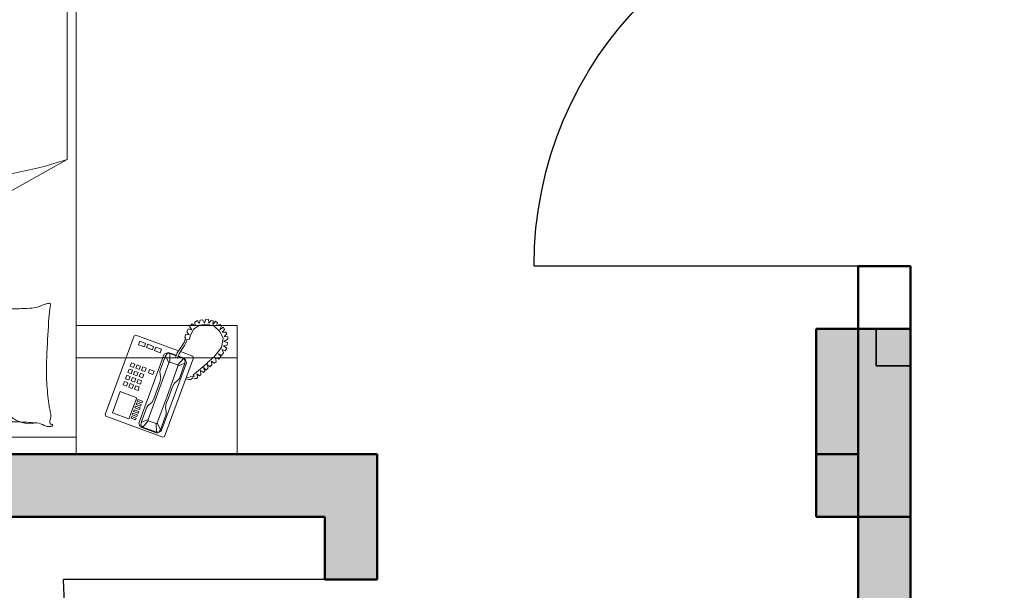
# Model space of a CAD drawing. Units: inches. Extents: x -7 to 1228, y -146 to 1091.
# Tile 75 of 88: x 722 to 816, y 835 to 890. Entities that reach past the tile are written whole.
import ezdxf

# ---------------------------------------------------------------- set-up
doc = ezdxf.new("R2010")
doc.units = ezdxf.units.IN
for name, color, linetype, lineweight in [('A-COLS', 6, 'Continuous', 35), ('A-DOOR', 4, 'Continuous', 25), ('A-FURN', 8, 'Continuous', 18), ('A-WALL', 7, 'Continuous', 50), ('A-WALL-PATT', 251, 'Continuous', 13)]:
    doc.layers.add(name, color=color, linetype=linetype, lineweight=lineweight)
doc.styles.add('DIM_FONT', font='SIMPLEX.shx', dxfattribs={"width": 0.8})

# ---------------------------------------------------------------- blocks, each defined once
blk = doc.blocks.new('A$C4F634EDD')
for p, q in [((0.5, 2.6295), (2.3, 2.6295)), ((2.3, 2.6295), (2.3, 0.5295)), ((2.3, 2.6295), (2.8, 2.6295)), ((2.3, 2.2295), (2.3, 2.6295)), ((2.8, 2.6295), (2.8, 2.2295)), ((0.5, 2.5771), (2.3, 2.5771)), ((2.392, 2.5115), (2.5692, 2.5765)), ((2.5692, 2.5765), (2.574, 2.5743)), ((2.574, 2.5743), (2.6638, 2.3298)), ((2.4946, 2.5331), (2.4985, 2.5445)), ((2.4985, 2.5445), (2.5516, 2.564)), ((2.5062, 2.5454), (2.5004, 2.5392)), ((2.5004, 2.5392), (2.5013, 2.5315)), ((2.5062, 2.5454), (2.5487, 2.561)), ((2.5235, 2.5256), (2.5062, 2.5454)), ((2.5483, 2.5347), (2.5487, 2.561)), ((2.5487, 2.561), (2.5571, 2.56)), ((2.5615, 2.5536), (2.5514, 2.5318)), ((2.5516, 2.564), (2.5637, 2.5584)), ((2.5571, 2.56), (2.5615, 2.5536)), ((2.5615, 2.5536), (2.5791, 2.5058)), ((2.5637, 2.5584), (2.6418, 2.3458)), ((2.3898, 2.5066), (2.392, 2.5115)), ((2.412, 2.5007), (2.4634, 2.5196)), ((2.4634, 2.5196), (2.4875, 2.454)), ((2.4842, 2.5232), (2.47, 2.518)), ((2.47, 2.518), (2.472, 2.5127)), ((2.472, 2.5127), (2.4862, 2.5179)), ((2.4881, 2.5126), (2.4739, 2.5074)), ((2.4862, 2.5179), (2.4842, 2.5232)), ((2.4901, 2.5073), (2.4881, 2.5126)), ((2.5734, 2.3187), (2.4946, 2.5331)), ((2.5013, 2.5315), (2.5188, 2.4836)), ((2.5013, 2.5315), (2.5231, 2.5214)), ((2.5231, 2.5214), (2.5235, 2.5256)), ((2.5523, 2.4417), (2.5231, 2.5214)), ((2.5483, 2.5347), (2.5235, 2.5256)), ((2.5514, 2.5318), (2.5483, 2.5347)), ((2.5807, 2.4521), (2.5514, 2.5318)), ((2.4795, 2.2621), (2.3898, 2.5066)), ((2.4361, 2.4352), (2.412, 2.5007)), ((2.4739, 2.5074), (2.4759, 2.502)), ((2.4759, 2.502), (2.4901, 2.5073)), ((2.492, 2.5019), (2.4778, 2.4967)), ((2.4778, 2.4967), (2.4798, 2.4914)), ((2.4798, 2.4914), (2.494, 2.4966)), ((2.4959, 2.4913), (2.4817, 2.4861)), ((2.4817, 2.4861), (2.4837, 2.4808)), ((2.4837, 2.4808), (2.4979, 2.486)), ((2.4998, 2.4807), (2.4856, 2.4755)), ((2.494, 2.4966), (2.492, 2.5019)), ((2.4979, 2.486), (2.4959, 2.4913)), ((2.5018, 2.4754), (2.4998, 2.4807)), ((2.5188, 2.4836), (2.5256, 2.4761)), ((2.5788, 2.4956), (2.5767, 2.4848)), ((2.5767, 2.4848), (2.5795, 2.4717)), ((2.5791, 2.5058), (2.5788, 2.4956)), ((2.4875, 2.454), (2.4361, 2.4352)), ((2.4856, 2.4755), (2.4876, 2.4702)), ((2.4876, 2.4702), (2.5018, 2.4754)), ((2.5037, 2.47), (2.4895, 2.4648)), ((2.4895, 2.4648), (2.4915, 2.4595)), ((2.4915, 2.4595), (2.5057, 2.4647)), ((2.5057, 2.4647), (2.5037, 2.47)), ((2.5256, 2.4761), (2.5342, 2.4692)), ((2.5342, 2.4692), (2.5405, 2.4574)), ((2.5405, 2.4574), (2.547, 2.4397)), ((2.5795, 2.4717), (2.586, 2.454)), ((2.5807, 2.4521), (2.6158, 2.3564)), ((2.5984, 2.4204), (2.586, 2.454)), ((2.4457, 2.4146), (2.4563, 2.4185)), ((2.4563, 2.4185), (2.4602, 2.4078)), ((2.4634, 2.4211), (2.474, 2.425)), ((2.4673, 2.4104), (2.4634, 2.4211)), ((2.474, 2.425), (2.4779, 2.4143)), ((2.4811, 2.4276), (2.4917, 2.4315)), ((2.485, 2.4169), (2.4811, 2.4276)), ((2.4956, 2.4208), (2.485, 2.4169)), ((2.4917, 2.4315), (2.4956, 2.4208)), ((2.5594, 2.4061), (2.547, 2.4397)), ((2.5523, 2.4417), (2.5875, 2.346)), ((2.6047, 2.4086), (2.5984, 2.4204)), ((2.4496, 2.4039), (2.4457, 2.4146)), ((2.4602, 2.4078), (2.4496, 2.4039)), ((2.4528, 2.3951), (2.4635, 2.399)), ((2.4567, 2.3844), (2.4528, 2.3951)), ((2.4674, 2.3883), (2.4567, 2.3844)), ((2.4635, 2.399), (2.4674, 2.3883)), ((2.4779, 2.4143), (2.4673, 2.4104)), ((2.4706, 2.4016), (2.4812, 2.4055)), ((2.4745, 2.3909), (2.4706, 2.4016)), ((2.4851, 2.3949), (2.4745, 2.3909)), ((2.4777, 2.3821), (2.4883, 2.386)), ((2.4812, 2.4055), (2.4851, 2.3949)), ((2.4883, 2.4081), (2.4989, 2.412)), ((2.4922, 2.3975), (2.4883, 2.4081)), ((2.4883, 2.386), (2.4922, 2.3754)), ((2.5028, 2.4014), (2.4922, 2.3975)), ((2.4954, 2.3886), (2.5061, 2.3925)), ((2.4993, 2.378), (2.4954, 2.3886)), ((2.4989, 2.412), (2.5028, 2.4014)), ((2.5061, 2.3925), (2.51, 2.3819)), ((2.5622, 2.393), (2.5594, 2.4061)), ((2.5601, 2.3822), (2.5622, 2.393)), ((2.6133, 2.4017), (2.6047, 2.4086)), ((2.6201, 2.3941), (2.6133, 2.4017)), ((2.6376, 2.3463), (2.6201, 2.3941)), ((2.6499, 2.3979), (2.6397, 2.3953)), ((2.6417, 2.39), (2.6488, 2.391)), ((2.6488, 2.391), (2.6538, 2.3895)), ((2.6551, 2.397), (2.6499, 2.3979)), ((2.6538, 2.3895), (2.6596, 2.388)), ((2.6627, 2.392), (2.6551, 2.397)), ((2.6596, 2.388), (2.6626, 2.3867)), ((2.6626, 2.3867), (2.6662, 2.388)), ((2.6692, 2.394), (2.6627, 2.392)), ((2.6662, 2.388), (2.6632, 2.3828)), ((2.6736, 2.3944), (2.6692, 2.394)), ((2.6765, 2.391), (2.6736, 2.3944)), ((2.6742, 2.3795), (2.6765, 2.391)), ((2.6824, 2.3858), (2.6742, 2.3795)), ((2.6873, 2.3815), (2.6824, 2.3858)), ((2.46, 2.3756), (2.4706, 2.3795)), ((2.4639, 2.365), (2.46, 2.3756)), ((2.4745, 2.3689), (2.4639, 2.365)), ((2.4672, 2.3561), (2.4778, 2.36)), ((2.4711, 2.3455), (2.4672, 2.3561)), ((2.4706, 2.3795), (2.4745, 2.3689)), ((2.4816, 2.3715), (2.4777, 2.3821)), ((2.4778, 2.36), (2.4817, 2.3494)), ((2.4922, 2.3754), (2.4816, 2.3715)), ((2.4849, 2.3626), (2.4955, 2.3665)), ((2.4888, 2.352), (2.4849, 2.3626)), ((2.4994, 2.3559), (2.4888, 2.352)), ((2.4955, 2.3665), (2.4994, 2.3559)), ((2.51, 2.3819), (2.4993, 2.378)), ((2.5026, 2.3691), (2.5132, 2.373)), ((2.5065, 2.3585), (2.5026, 2.3691)), ((2.5171, 2.3624), (2.5065, 2.3585)), ((2.5132, 2.373), (2.5171, 2.3624)), ((2.5238, 2.3769), (2.538, 2.3821)), ((2.5277, 2.3663), (2.5238, 2.3769)), ((2.5419, 2.3715), (2.5277, 2.3663)), ((2.538, 2.3821), (2.5419, 2.3715)), ((2.5598, 2.372), (2.5601, 2.3822)), ((2.5774, 2.3242), (2.5598, 2.372)), ((2.6158, 2.3564), (2.6154, 2.3522)), ((2.6376, 2.3463), (2.6158, 2.3564)), ((2.6632, 2.3828), (2.6736, 2.3744)), ((2.6736, 2.3744), (2.6922, 2.3593)), ((2.6853, 2.369), (2.6873, 2.3815)), ((2.6946, 2.376), (2.6853, 2.369)), ((2.6922, 2.3593), (2.7051, 2.3473)), ((2.6995, 2.3713), (2.6946, 2.376)), ((2.695, 2.3603), (2.6995, 2.3713)), ((2.7031, 2.3682), (2.695, 2.3603)), ((2.7096, 2.3616), (2.7031, 2.3682)), ((2.7062, 2.351), (2.7096, 2.3616)), ((2.7147, 2.3578), (2.7062, 2.351)), ((2.7214, 2.3517), (2.7147, 2.3578)), ((2.8, 2.3301), (2.3, 2.3301)), ((2.4817, 2.3494), (2.4711, 2.3455)), ((2.5774, 2.3242), (2.5875, 2.346)), ((2.5875, 2.346), (2.5905, 2.3431)), ((2.5905, 2.3431), (2.5901, 2.3168)), ((2.6154, 2.3522), (2.5905, 2.3431)), ((2.613, 2.3312), (2.6077, 2.3293)), ((2.6077, 2.3293), (2.6135, 2.3141)), ((2.6192, 2.3174), (2.613, 2.3312)), ((2.6153, 2.3261), (2.6327, 2.3324)), ((2.6154, 2.3522), (2.6327, 2.3324)), ((2.6369, 2.332), (2.6161, 2.3243)), ((2.6616, 2.3249), (2.6234, 2.3109)), ((2.6327, 2.3324), (2.6385, 2.3386)), ((2.6418, 2.3458), (2.6369, 2.332)), ((2.6385, 2.3386), (2.6376, 2.3463)), ((2.6638, 2.3298), (2.6616, 2.3249)), ((2.7051, 2.3473), (2.7079, 2.3475)), ((2.7079, 2.3475), (2.7079, 2.3443)), ((2.7079, 2.3443), (2.727, 2.3277)), ((2.7196, 2.34), (2.7214, 2.3517)), ((2.7286, 2.3466), (2.7196, 2.34)), ((2.727, 2.3277), (2.7512, 2.2983)), ((2.7346, 2.3423), (2.7286, 2.3466)), ((2.732, 2.3295), (2.7346, 2.3423)), ((2.7423, 2.3345), (2.732, 2.3295)), ((2.7406, 2.3172), (2.7495, 2.325)), ((2.7495, 2.325), (2.7423, 2.3345)), ((2.6172, 2.3086), (2.4844, 2.2599)), ((2.5114, 2.2959), (2.4936, 2.2894)), ((2.5153, 2.2853), (2.5114, 2.2959)), ((2.5362, 2.305), (2.5185, 2.2985)), ((2.5185, 2.2985), (2.5224, 2.2879)), ((2.5224, 2.2879), (2.5401, 2.2944)), ((2.5401, 2.2944), (2.5362, 2.305)), ((2.561, 2.3141), (2.5433, 2.3076)), ((2.5433, 2.3076), (2.5472, 2.297)), ((2.5472, 2.297), (2.5649, 2.3035)), ((2.5649, 2.3035), (2.561, 2.3141)), ((2.5855, 2.3131), (2.5734, 2.3187)), ((2.5818, 2.3178), (2.5774, 2.3242)), ((2.5901, 2.3168), (2.5818, 2.3178)), ((2.6104, 2.3222), (2.5855, 2.3131)), ((2.5901, 2.3168), (2.6097, 2.324)), ((2.6135, 2.3141), (2.6244, 2.2977)), ((2.626, 2.3069), (2.6192, 2.3174)), ((2.6244, 2.2977), (2.6349, 2.2825)), ((2.6365, 2.2916), (2.626, 2.3069)), ((2.7519, 2.3218), (2.7406, 2.3172)), ((2.7512, 2.2983), (2.756, 2.2695)), ((2.7575, 2.3144), (2.7519, 2.3218)), ((2.7526, 2.3045), (2.7575, 2.3144)), ((2.7622, 2.308), (2.7526, 2.3045)), ((2.7574, 2.2924), (2.7673, 2.2997)), ((2.7673, 2.2997), (2.7622, 2.308)), ((2.4936, 2.2894), (2.4976, 2.2788)), ((2.4976, 2.2788), (2.5153, 2.2853)), ((2.6349, 2.2825), (2.638, 2.273)), ((2.6407, 2.2834), (2.6365, 2.2916)), ((2.6399, 2.2712), (2.6374, 2.2659)), ((2.6374, 2.2659), (2.6398, 2.257)), ((2.638, 2.273), (2.6399, 2.2712)), ((2.6438, 2.2739), (2.6407, 2.2834)), ((2.6519, 2.2716), (2.6438, 2.2739)), ((2.6535, 2.2628), (2.6519, 2.2716)), ((2.756, 2.2695), (2.7459, 2.2483)), ((2.7687, 2.2905), (2.7574, 2.2924)), ((2.7587, 2.279), (2.7699, 2.2828)), ((2.7708, 2.2725), (2.7587, 2.279)), ((2.759, 2.2637), (2.7706, 2.2643)), ((2.7676, 2.2559), (2.759, 2.2637)), ((2.7699, 2.2828), (2.7687, 2.2905)), ((2.7706, 2.2643), (2.7708, 2.2725)), ((2.4844, 2.2599), (2.4795, 2.2621)), ((2.6398, 2.257), (2.6509, 2.259)), ((2.6509, 2.259), (2.6431, 2.2492)), ((2.6431, 2.2492), (2.6473, 2.2398)), ((2.6473, 2.2398), (2.6592, 2.2429)), ((2.6592, 2.2429), (2.6521, 2.2314)), ((2.6636, 2.2409), (2.6535, 2.2628)), ((2.6836, 2.2287), (2.6636, 2.2409)), ((2.7459, 2.2483), (2.7284, 2.2317)), ((2.7509, 2.2314), (2.7459, 2.2418)), ((2.7459, 2.2418), (2.7568, 2.2352)), ((2.7529, 2.2505), (2.7645, 2.2498)), ((2.7607, 2.2424), (2.7529, 2.2505)), ((2.7568, 2.2352), (2.7607, 2.2424)), ((2.7645, 2.2498), (2.7676, 2.2559)), ((2.8, 2.2295), (2.3, 2.2295)), ((2.6521, 2.2314), (2.6598, 2.2248)), ((2.6598, 2.2248), (2.6697, 2.2309)), ((2.6697, 2.2309), (2.6684, 2.219)), ((2.6684, 2.219), (2.6761, 2.2145)), ((2.6761, 2.2145), (2.6821, 2.2237)), ((2.6821, 2.2237), (2.6843, 2.2135)), ((2.7063, 2.2256), (2.6836, 2.2287)), ((2.6843, 2.2135), (2.6927, 2.2117)), ((2.6927, 2.2117), (2.6986, 2.222)), ((2.6986, 2.222), (2.7019, 2.2098)), ((2.7019, 2.2098), (2.7102, 2.2104)), ((2.7284, 2.2317), (2.7063, 2.2256)), ((2.7102, 2.2104), (2.7113, 2.2218)), ((2.7113, 2.2218), (2.7192, 2.2137)), ((2.7192, 2.2137), (2.7255, 2.2152)), ((2.7255, 2.2152), (2.7242, 2.2265)), ((2.7242, 2.2265), (2.7324, 2.2165)), ((2.7324, 2.2165), (2.7386, 2.2208)), ((2.7386, 2.2208), (2.7354, 2.2306)), ((2.7354, 2.2306), (2.7462, 2.2264)), ((2.7462, 2.2264), (2.7509, 2.2314)), ((1.5035, 2.141), (2.2716, 1.7136)), ((2.2716, 0.5617), (2.2716, 1.7136))]:
    blk.add_line(p, q)
for centre, radius, start, end in [((2.1724, 2.5864), 0.0539, 275.2592, 300.6513), ((2.2146, 2.5152), 0.0289, 85.6975, 120.6513), ((2.2149, 2.519), 0.0251, 68.2117, 85.6975), ((2.224, 2.5395), 0.00232, 258.1069, 19.564), ((2.2229, 2.5391), 0.00342, 19.564, 68.2117), ((2.0797, 4.0232), 1.4943, 269.4243, 271.9079), ((2.1588, 2.4357), 0.0992, 105.9352, 126.0864), ((2.1021, 3.3501), 0.8208, 271.9079, 275.2592), ((2.1588, 2.4357), 0.0992, 85.7841, 105.9352), ((2.2331, 2.5288), 0.0156, 158.0096, 201.421), ((2.2226, 2.533), 0.00428, 78.1069, 158.0096), ((2.1881, 2.5111), 0.0328, 351.8665, 21.421), ((2.4114, 2.448), 0.1983, 167.8905, 172.3191), ((1.977, 2.5413), 0.246, 347.8905, 351.8665), ((3.1198, 2.3525), 0.9131, 172.3191, 176.6313), ((2.8858, 2.3663), 0.6787, 176.6313, 181.6331), ((3.5721, 2.3859), 1.3652, 181.6331, 183.055), ((15.8249, 3.0398), 13.6356, 183.05496, 183.50486), ((2.5355, 2.2258), 0.3212, 183.5049, 189.9984), ((2.0833, 1.0141), 1.164, 86.426, 89.7135), ((2.1467, 2.0302), 0.1459, 77.131, 86.426), ((2.1691, 2.1283), 0.0453, 62.7159, 77.131), ((2.2251, 2.2367), 0.0767, 242.7159, 253.7788), ((2.2281, 2.247), 0.0875, 253.7788, 262.8796), ((2.2174, 2.1615), 0.00132, 262.8796, 343.3022), ((2.2001, 2.1667), 0.0193, 343.3022, 9.9984), ((1.2737, -2.2227), 4.0646, 77.0745, 79.2724), ((2.0359, 1.0981), 0.6574, 74.0648, 77.0745), ((1.7125, -0.0344), 1.8351, 72.2636, 74.0648)]:
    blk.add_arc(centre, radius, start, end)
at = {"style": 'DIM_FONT', "width": 0.8, "flags": 9}
for tag, p in [('YSIZE', (0.5, 2.6295)), ('XSIZE', (0.5, 2.6295)), ('XSIZE', (2.2985, 2.6295)), ('YSIZE', (2.2985, 2.6295))]:
    blk.add_attdef(tag, p, '', height=0.0005, dxfattribs=at)
blk = doc.blocks.new('DOOR-750')
blk.add_line((30, 30), (30, 0))
blk.add_arc((30, 30), 30, 180, 270)
blk = doc.blocks.new('DOOR-900')
blk.add_line((36, 0), (36, 36))
blk.add_arc((36, 0), 36, 90, 180)

msp = doc.modelspace()

# ---------------------------------------------------------------- hatches: boundary and pattern name
at = {"layer": 'A-COLS'}
h = msp.add_hatch(color=256, dxfattribs=at)
h.dxf.hatch_style = 1
h.paths.add_polyline_path([(807, 856.454), (803.711, 856.454), (803.711, 860), (798, 860), (798, 842), (807, 842)])
h = msp.add_hatch(color=256, dxfattribs=at)
h.dxf.hatch_style = 1
h.paths.add_polyline_path([(807, 856.454), (807, 860), (803.711, 860), (803.711, 856.454)])
at = {"layer": 'A-WALL-PATT'}
h = msp.add_hatch(color=256, dxfattribs=at)
h.dxf.hatch_style = 1
h.paths.add_polyline_path([(69, 568), (60, 568), (60, 493), (63.289, 493), (69, 493)])
h.paths.add_polyline_path([(69, 662.405), (60, 662.405), (60, 586), (69, 586)], flags=17)
h.paths.add_polyline_path([(69, 723), (184, 723), (184, 734), (179, 734), (179, 728), (69, 728), (69, 741.623), (60, 741.623), (60, 698.405), (69, 698.405)], flags=17)
h.paths.add_polyline_path([(69, 782), (231, 782), (231, 728), (231, 723), (231, 586), (236, 586), (236, 787), (69, 787), (69, 800.126), (60, 800.126), (60, 765.623), (69, 765.623)])
h.paths.add_polyline_path([(184, 842), (189, 842), (189, 848), (173, 848), (173, 842), (179, 842), (179, 787), (184, 787)])
h.paths.add_polyline_path([(118.22, 69), (69, 69), (69, 60), (118.22, 60)])
h.paths.add_polyline_path([(227, 69), (154.22, 69), (154.22, 60), (227, 60)])
h.paths.add_polyline_path([(236, 60), (232.711, 60), (227, 60), (227, 36), (236, 36)])
h.paths.add_polyline_path([(389, 60), (380, 60), (380, 36), (389, 36)])
h.paths.add_polyline_path([(384, 181), (380, 181), (380, 115), (380, 78), (384, 78)])
h.paths.add_polyline_path([(380, 115), (334.547, 115), (334.547, 109), (380, 109)])
h.paths.add_polyline_path([(274.547, 115), (236, 115), (236, 201), (232.711, 201), (231, 201), (231, 78), (236, 78), (236, 109), (274.547, 109)])
h.paths.add_polyline_path([(69, 123), (60, 123), (60, 78), (69, 78)])
h.paths.add_polyline_path([(69, 201), (60, 201), (60, 159), (69, 159)])
h.paths.add_polyline_path([(143, 219), (69, 219), (69, 213), (143, 213)], flags=17)
h.paths.add_polyline_path([(189, 219), (184, 219), (184, 274), (231, 274), (231, 219), (236, 219), (236, 279), (184, 279), (184, 297), (179, 297), (179, 279), (69, 279), (69, 290.912), (60, 290.912), (60, 262.179), (69, 262.179), (69, 274), (179, 274), (179, 219), (173, 219), (173, 213), (189, 213)])
h.paths.add_polyline_path([(69, 238.179), (60, 238.179), (60, 219), (69, 219)], flags=17)
h.paths.add_polyline_path([(69, 333), (60, 333), (60, 314.912), (69, 314.912), (69, 316.965)])
h.paths.add_polyline_path([(190, 338), (184, 338), (69, 338), (69, 333), (179, 333), (179, 327), (184, 327), (184, 333.021), (190, 333.046)])
h.paths.add_polyline_path([(69, 386.806), (60, 386.806), (60, 351), (69, 351)])
h.paths.add_polyline_path([(69, 475), (60, 475), (60, 422.806), (69, 422.806)])
h.paths.add_polyline_path([(236, 475), (231, 475), (231, 351.238), (236, 351.238)])
h.paths.add_polyline_path([(384, 475), (380, 475), (380, 362), (384, 362)])
h.paths.add_polyline_path([(547, 307), (439, 307), (439, 356), (445, 356), (445, 362), (433, 362), (433, 307), (380, 307), (380, 244), (380, 241), (384, 241), (384, 301), (433, 301), (433, 277), (439, 277), (439, 301), (547, 301)])
h.paths.add_polyline_path([(547, 241), (439, 241), (439, 247), (433, 247), (433, 235), (547, 235)])
h.paths.add_polyline_path([(450, 69), (440.286, 69), (424.889, 69), (389, 69), (389, 60), (450, 60)])
h.paths.add_polyline_path([(547, 69), (486, 69), (486, 60), (547, 60)])
h.paths.add_polyline_path([(556, 148.268), (547, 148.268), (547, 78), (556, 78)])
h.paths.add_polyline_path([(556, 223), (547, 223), (547, 195), (547, 184.268), (556, 184.268)])
h.paths.add_polyline_path([(556, 311.192), (547, 311.192), (547, 273.075), (556, 273.075)])
h.paths.add_polyline_path([(556, 344), (552.711, 344), (547, 344), (547, 335.192), (556, 335.192)])
h.paths.add_polyline_path([(556, 249.075), (547, 249.075), (547, 241), (556, 241)])
h.paths.add_polyline_path([(547, 362), (475, 362), (475, 356), (547, 356)], flags=0)
h.paths.add_polyline_path([(556, 399.621), (547, 399.621), (547, 362), (556, 362)])
h.paths.add_polyline_path([(556, 475), (547, 475), (547, 435.621), (556, 435.621)])
h.paths.add_polyline_path([(547, 493), (389, 493), (389, 487), (547, 487)])
h.paths.add_polyline_path([(380, 493), (278, 493), (278, 487), (380, 487)])
h.paths.add_polyline_path([(227, 493), (69, 493), (69, 487), (227, 487)])
h.paths.add_polyline_path([(643, 122.445), (634, 122.445), (634, 78), (643, 78)])
h.paths.add_polyline_path([(702.5, 69), (692.786, 69), (677.389, 69), (643, 69), (643, 60), (702.5, 60)])
h.paths.add_polyline_path([(798, 69), (738.5, 69), (738.5, 60), (798, 60)])
h.paths.add_polyline_path([(807, 60), (803.711, 60), (798, 60), (798, 36), (807, 36)])
h.paths.add_polyline_path([(807, 109), (846.751, 109), (846.751, 115), (807, 115), (807, 159), (802, 159), (802, 78), (807, 78)])
h.paths.add_polyline_path([(807, 201), (802, 201), (802, 195), (807, 195)])
h.paths.add_polyline_path([(643, 201), (634, 201), (634, 158.445), (643, 158.445)])
h.paths.add_polyline_path([(756, 225), (751, 225), (751, 219), (643, 219), (643, 213), (756, 213)])
h.paths.add_polyline_path([(643, 240.848), (634, 240.848), (634, 219), (643, 219)])
h.paths.add_polyline_path([(643, 274), (643, 288.629), (634, 288.629), (634, 264.848), (643, 264.848)])
h.paths.add_polyline_path([(802, 279), (756, 279), (756, 297), (751, 297), (751, 279), (643, 279), (643, 274), (751, 274), (751, 255), (756, 255), (756, 274), (802, 274)])
h.paths.add_polyline_path([(807, 333), (803.711, 333), (802, 333), (802, 279), (802, 274), (802, 219), (807, 219)])
h.paths.add_polyline_path([(956, 182), (951, 182), (951, 115), (906.751, 115), (906.751, 109), (951, 109), (951, 78), (956, 78)])
h.paths.add_polyline_path([(960, 60), (951, 60), (951, 36), (960, 36)])
h.paths.add_polyline_path([(1021, 69), (1005.781, 69), (960, 69), (960, 60), (1021, 60)])
h.paths.add_polyline_path([(956, 224), (951, 224), (951, 218), (956, 218)])
h.paths.add_polyline_path([(956, 302), (1004, 302), (1004, 278), (1010, 278), (1010, 302), (1118, 302), (1118, 290.809), (1127, 290.809), (1127, 326.968), (1118, 326.968), (1118, 320.966), (1118, 307), (1010, 307), (1010, 356), (1016, 356), (1016, 362), (1004, 362), (1004, 307), (951, 307), (951, 244), (951, 242), (954.289, 242), (956, 242)])
h.paths.add_polyline_path([(643, 333), (634, 333), (634, 312.629), (643, 312.629), (643, 316.965)])
h.paths.add_polyline_path([(756, 338), (643, 338), (643, 333), (751, 333), (751, 327), (756, 327)])
h.paths.add_polyline_path([(643, 388), (634, 388), (634, 351), (643, 351)])
h.paths.add_polyline_path([(807, 357), (802, 357), (802, 351), (807, 351)])
h.paths.add_polyline_path([(807, 475), (802, 475), (802, 393), (807, 393)])
h.paths.add_polyline_path([(643, 475), (634, 475), (634, 424), (643, 424)])
h.paths.add_polyline_path([(798, 493), (643, 493), (643, 487), (798, 487)])
h.paths.add_polyline_path([(634, 493), (556, 493), (556, 487), (634, 487)])
h.paths.add_polyline_path([(813, 493), (807, 493), (807, 487), (813, 487)])
h.paths.add_polyline_path([(951, 493), (849, 493), (849, 487), (951, 487)])
h.paths.add_polyline_path([(956, 484), (951, 484), (951, 374), (956, 374)])
h.paths.add_polyline_path([(1109, 493), (969, 493), (969, 487), (1109, 487)])
h.paths.add_polyline_path([(1127, 484), (1118, 484), (1118, 450.641), (1127, 450.641)])
h.paths.add_polyline_path([(1127, 414.641), (1118, 414.641), (1118, 365), (1127, 365)])
h.paths.add_polyline_path([(1109, 362), (1046, 362), (1046, 356), (1109, 356)], flags=17)
h.paths.add_polyline_path([(1127, 356), (1123.454, 356), (1118, 356), (1118, 350.968), (1127, 350.968)], flags=0)
h.paths.add_polyline_path([(1127, 266.809), (1118, 266.809), (1118, 262.361), (1118, 242), (1127, 242)], flags=17)
h.paths.add_polyline_path([(1118, 242), (1010, 242), (1010, 248), (1004, 248), (1004, 237), (1118, 237)])
h.paths.add_polyline_path([(1127, 224), (1118, 224), (1118, 170), (1127, 170)])
h.paths.add_polyline_path([(1127, 134), (1118, 134), (1118, 78), (1127, 78)])
h.paths.add_polyline_path([(1118, 69), (1057, 69), (1057, 60), (1118, 60)])
h.paths.add_polyline_path([(227, 571.546), (227, 574), (69, 574), (69, 568), (227, 568)])
h.paths.add_polyline_path([(380, 571.546), (380, 574), (278, 574), (278, 568), (380, 568)])
h.paths.add_polyline_path([(242, 574), (236, 574), (236, 568), (242, 568)])
h.paths.add_polyline_path([(547, 571.546), (547, 574), (389, 574), (389, 568), (547, 568)])
h.paths.add_polyline_path([(384, 733), (380, 733), (380, 586), (384, 586)])
h.paths.add_polyline_path([(556, 646), (634, 646), (634, 655), (547, 655), (547, 586), (556, 586)])
h.paths.add_polyline_path([(634, 574), (556, 574), (556, 568), (634, 568)])
h.paths.add_polyline_path([(643, 655), (634, 655), (634, 586), (643, 586)])
h.paths.add_polyline_path([(798, 574), (643, 574), (643, 568), (798, 568)])
h.paths.add_polyline_path([(643, 663.854), (634, 663.854), (634, 655), (643, 655)])
h.paths.add_polyline_path([(556, 676.967), (547, 676.967), (547, 655), (556, 655)])
h.paths.add_polyline_path([(556, 733), (547, 733), (547, 712.967), (556, 712.967)])
h.paths.add_polyline_path([(643, 710), (634, 710), (634, 699.854), (643, 699.854)])
h.paths.add_polyline_path([(807, 668), (802, 668), (802, 586), (807, 586)])
h.paths.add_polyline_path([(951, 574), (849, 574), (849, 568), (951, 568)])
h.paths.add_polyline_path([(956, 691), (951, 691), (951, 577), (956, 577)])
h.paths.add_polyline_path([(1109, 574), (969, 574), (969, 568), (1109, 568)])
h.paths.add_polyline_path([(1127, 643.403), (1118, 643.403), (1118, 577), (1127, 577)])
h.paths.add_polyline_path([(1127, 568), (1123.454, 568), (1118, 568), (1118, 493), (1127, 493)])
h.paths.add_polyline_path([(1127, 733), (1118, 733), (1118, 679.403), (1127, 679.403)])
h.paths.add_polyline_path([(1127, 777.348), (1118, 777.348), (1118, 770.035), (1118, 751), (1127, 751)], flags=17)
h.paths.add_polyline_path([(1118, 751), (1010, 751), (1010, 757), (1004, 757), (1004, 745), (1118, 745)])
h.paths.add_polyline_path([(956, 811), (1004, 811), (1004, 787), (1010, 787), (1010, 811), (1017.874, 811), (1017.874, 811.627, -0.414214), (1018.247, 812), (1031.978, 812, -0.414214), (1032.351, 811.627), (1032.351, 811), (1118, 811), (1118, 801.348), (1127, 801.348), (1127, 834.685), (1118, 834.685), (1118, 830.238), (1118, 817), (1010, 817), (1010, 866), (1016, 866), (1016, 872), (1004, 872), (1004, 817), (956, 817), (956, 866), (951, 866), (951, 751), (954.289, 751), (956, 751)])
h.paths.add_polyline_path([(1118, 872), (1046, 872), (1046, 866), (1118, 866)], flags=17)
h.paths.add_polyline_path([(1127, 924.711), (1118, 924.711), (1118, 884), (1127, 884)])
h.paths.add_polyline_path([(1127, 866), (1123.711, 866), (1118, 866), (1118, 858.685), (1127, 858.685)], flags=17)
h.paths.add_polyline_path([(956, 983), (951, 983), (951, 952), (807, 952), (807, 983), (802, 983), (802, 902), (807, 902), (807, 946), (951, 946), (951, 884), (956, 884)])
h.paths.add_polyline_path([(807, 842), (802, 842), (802, 787), (756, 787), (756, 806), (751, 806), (751, 787), (643, 787), (643, 782), (751, 782), (751, 764), (756, 764), (756, 782), (802, 782), (802, 728), (807, 728)])
h.paths.add_polyline_path([(756, 848), (643, 848), (643, 842), (751, 842), (751, 836), (756, 836)])
h.paths.add_polyline_path([(756, 734), (751, 734), (751, 728), (643, 728), (643, 723), (756, 723)])
h.paths.add_polyline_path([(643, 749.791), (634, 749.791), (634, 728), (637.289, 728), (643, 728)])
h.paths.add_polyline_path([(643, 805.405), (634, 805.405), (634, 773.791), (643, 773.791)])
h.paths.add_polyline_path([(643, 896.663), (634, 896.663), (634, 860), (637.289, 860), (643, 860)])
h.paths.add_polyline_path([(643, 842), (634, 842), (634, 829.405), (643, 829.405)])
h.paths.add_polyline_path([(643, 983), (634, 983), (634, 932.663), (643, 932.663)])
h.paths.add_polyline_path([(1127, 983), (1118, 983), (1118, 960.711), (1127, 960.711)])
h.paths.add_polyline_path([(1118, 1001), (1077.525, 1001), (1077.525, 992), (1118, 992)])
h.paths.add_polyline_path([(1041.525, 1001), (960, 1001), (960, 992), (1041.525, 992)])
h.paths.add_polyline_path([(960, 1025), (951, 1025), (951, 1001), (954.289, 1001), (960, 1001)])
h.paths.add_polyline_path([(807, 1025), (798, 1025), (798, 1001), (807, 1001)])
h.paths.add_polyline_path([(798, 1001), (738.5, 1001), (738.5, 992), (798, 992)])
h.paths.add_polyline_path([(702.5, 1001), (643, 1001), (643, 992), (702.5, 992)])
h.paths.add_polyline_path([(547, 1001), (499.113, 1001), (499.113, 992), (547, 992)])
h.paths.add_polyline_path([(463.113, 1001), (389, 1001), (389, 992), (463.113, 992)])
h.paths.add_polyline_path([(389, 1025), (380, 1025), (380, 1022), (380, 1001), (383.289, 1001), (389, 1001)])
h.paths.add_polyline_path([(236, 1025), (227, 1025), (227, 1001), (236, 1001)])
h.paths.add_polyline_path([(236, 983), (231, 983), (231, 860), (236, 860)])
h.paths.add_polyline_path([(274.547, 952), (236, 952), (236, 946), (274.547, 946)])
h.paths.add_polyline_path([(380, 952), (334.547, 952), (334.547, 946), (380, 946)])
h.paths.add_polyline_path([(384, 983), (380, 983), (380, 884), (383.289, 884), (384, 884)])
h.paths.add_polyline_path([(227, 1001), (155.012, 1001), (155.012, 992), (162.875, 992), (227, 992)])
h.paths.add_polyline_path([(119.012, 1001), (69, 1001), (69, 992), (119.012, 992)])
h.paths.add_polyline_path([(69, 983), (60, 983), (60, 922.987), (69, 922.987)])
h.paths.add_polyline_path([(69, 886.987), (60, 886.987), (60, 860), (63.289, 860), (69, 860)])
h.paths.add_polyline_path([(143, 848), (69, 848), (69, 842), (143, 842)])

# ---------------------------------------------------------------- linework, layer by layer
at = {"layer": 'A-COLS'}
msp.add_lwpolyline([(807, 860), (803.711, 860), (803.711, 856.454), (807, 856.454)], close=True, dxfattribs=at)
at = {"layer": 'A-WALL'}
for p, q in [((807, 866), (802, 866)), ((802, 866), (802, 848)), ((802, 787), (802, 866)), ((807, 866), (807, 704)), ((807, 704), (807, 866)), ((807, 860), (798, 860)), ((798, 860), (798, 842)), ((807, 860), (802, 860)), ((807, 842), (807, 860)), ((756, 848), (643, 848)), ((756, 848), (756, 836)), ((802, 848), (798, 848)), ((751, 842), (643, 842)), ((751, 842), (751, 836)), ((802, 842), (798, 842)), ((798, 842), (807, 842)), ((802, 842), (802, 787)), ((756, 836), (751, 836))]:
    msp.add_line(p, q, dxfattribs=at)

# ---------------------------------------------------------------- block references
at = {"layer": 'A-DOOR', "extrusion": (0, 0, -1), "zscale": -1}
for name, p, rotation in [('DOOR-900', (-807, 902), 269.9999999999997), ('DOOR-750', (-726, 806), 90)]:
    msp.add_blockref(name, p, dxfattribs=dict(at, rotation=rotation))
at = {"layer": 'A-FURN', "xscale": -30.79356024027943, "yscale": 30.79356024027943, "zscale": 30.79356024027943, "rotation": 180}
msp.add_blockref('A$C4F634EDD', (656.389, 928.972), dxfattribs=at)

doc.saveas('drawing.dxf')
